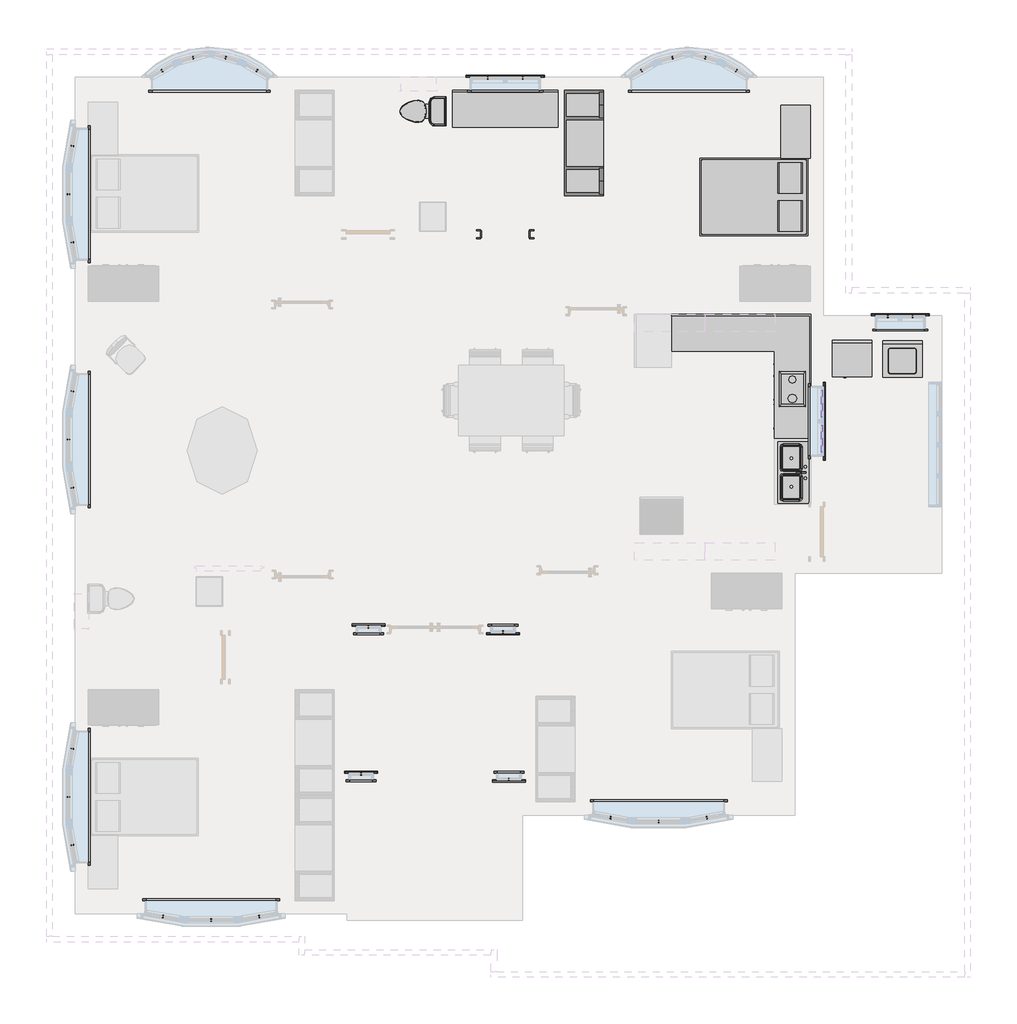
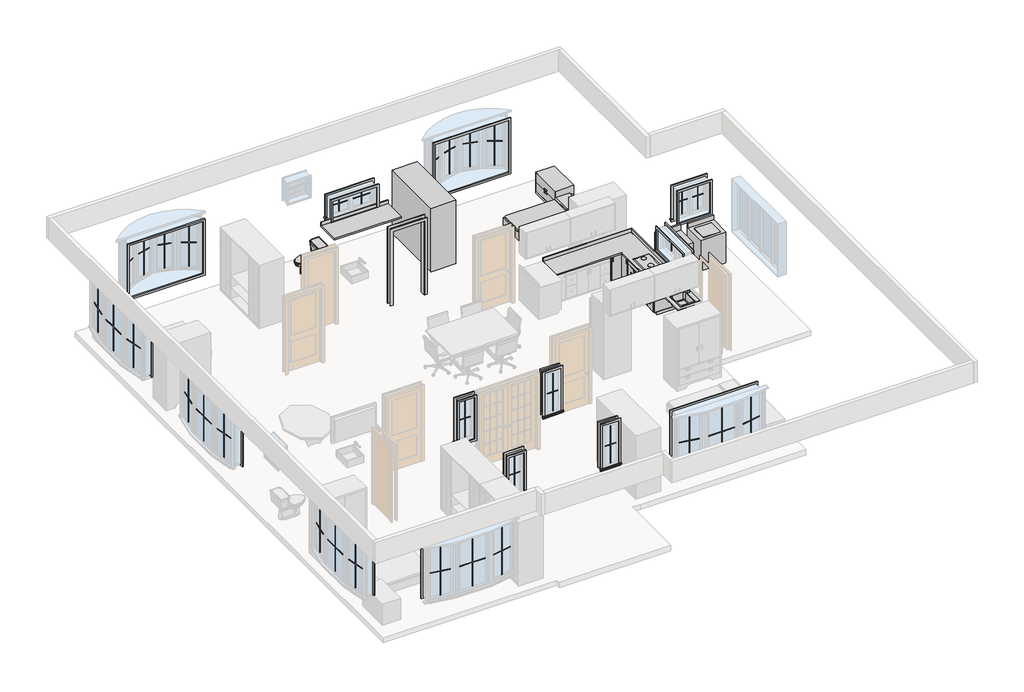
# One storey, part 2 of 2: 58 proxies, 7 furniture elements, 2 flow terminals.
"""IFC4 building model written with IfcOpenShell, lengths in millimetres."""

from ifc_helpers import new_model, si_unit, origin, place, context, project, spatial, transform, mapped, element, save
from components import proxy_3c1fa1d0, proxy_97c73763, muntin_pattern_2x2_muntin_pattern_2x2_d8607f27, muntin_pattern_2x2_muntin_pattern_2x2_395d1e8c, muntin_pattern_2x2_muntin_pattern_2x2_f815d33b, muntin_pattern_2x2_muntin_pattern_2x2_6cb77f41, muntin_pattern_2x2_muntin_pattern_2x2_7d820091, muntin_pattern_2x2_muntin_pattern_2x2_d662aa9d, muntin_pattern_2x2_muntin_pattern_2x2_3e0ecaf2, muntin_pattern_2x2_muntin_pattern_2x2_b3fe6957, muntin_pattern_2x2_muntin_pattern_2x2_0e1f1e2d, proxy_dc468f74, trim_window_exterior_flat_with_sill_a633738d, trim_window_exterior_flat_with_sill_f2223f96, trim_window_exterior_flat_with_sill_499ee38d, trim_window_interior_flat_picture_frame_9ca7b173, trim_window_interior_flat_picture_frame_fb3c0359, trim_window_interior_flat_picture_frame_0870d947, trim_window_interior_flat_picture_frame_1c9020d0, trim_window_interior_flat_picture_frame_a70901f7, proxy_e75280ca, flow_terminal_a53be723, toilet_domestic_3d_toilet_domestic_3d_ba6479b0, toilet_domestic_3d_toilet_domestic_3d_30431060, furniture_b04c6994, furniture_ff3c2f57, furniture_b58f7881, furniture_6b884072, furniture_6990e744, furniture_a71f50c7, furniture_88072bd9

model = new_model("IFC4")

# Units and contexts
model_context = context("Model", 3, world=origin())
ifc_project = project(units=[si_unit("LENGTHUNIT", "METRE", prefix="MILLI")], contexts=[model_context])

# Site, building, storey
site = spatial("IfcSite", under=ifc_project)
building = spatial("IfcBuilding", under=site)
storey = spatial("IfcBuildingStorey", under=building, Elevation=914.4)

# Proxies
placement = place(None, origin())
proxy_shape = proxy_3c1fa1d0(model_context)
element("IfcBuildingElementProxy", 1, Name="Cook Top-2 Unit : 12\" x 18\" 2", ObjectType="Cook Top-2 Unit : 12\" x 18\" 2", at=placement, inside=storey, context=model_context, shape_type="MappedRepresentation", body=[
    mapped(proxy_shape, transform((-7640.9494093, 9917.3485443, 914.4), x_axis=(-1.0, 0.0, 0.0), y_axis=(0.0, -1.0, 0.0), z_axis=(0.0, 0.0, 1.0))),
])
proxy_2_shape = proxy_97c73763(model_context)
element("IfcBuildingElementProxy", 2, Name="Dryer : 27\" x 25\" x 35\"", ObjectType="Dryer : 27\" x 25\" x 35\"", at=placement, inside=storey, context=model_context, shape_type="MappedRepresentation", body=[
    mapped(proxy_2_shape, transform((-7061.0868656, 10105.8627449, 914.4), x_axis=(1.0, 0.0, 0.0), y_axis=(0.0, 1.0, 0.0), z_axis=(0.0, 0.0, 1.0))),
])
muntin_pattern_2x2_muntin_pattern_2x2_shape = muntin_pattern_2x2_muntin_pattern_2x2_d8607f27(model_context)
element("IfcBuildingElementProxy", 3, Name="Muntin Pattern_2x2 : Muntin Pattern_2x2", ObjectType="Muntin Pattern_2x2 : Muntin Pattern_2x2", at=placement, inside=storey, context=model_context, shape_type="MappedRepresentation", body=[
    mapped(muntin_pattern_2x2_muntin_pattern_2x2_shape, transform((-20280.6244093, 13268.4987487, 1644.65), x_axis=(0.0, 1.0, 0.0), y_axis=(-1.0, 0.0, 0.0), z_axis=(0.0, 0.0, 1.0))),
])
element("IfcBuildingElementProxy", 4, Name="Muntin Pattern_2x2 : Muntin Pattern_2x2", ObjectType="Muntin Pattern_2x2 : Muntin Pattern_2x2", at=placement, inside=storey, context=model_context, shape_type="MappedRepresentation", body=[
    mapped(muntin_pattern_2x2_muntin_pattern_2x2_shape, transform((-20280.6244093, 9010.8237487, 1644.65), x_axis=(0.0, 1.0, 0.0), y_axis=(-1.0, 0.0, 0.0), z_axis=(0.0, 0.0, 1.0))),
])
element("IfcBuildingElementProxy", 5, Name="Muntin Pattern_2x2 : Muntin Pattern_2x2", ObjectType="Muntin Pattern_2x2 : Muntin Pattern_2x2", at=placement, inside=storey, context=model_context, shape_type="MappedRepresentation", body=[
    mapped(muntin_pattern_2x2_muntin_pattern_2x2_shape, transform((-20280.6244093, 2810.0487487, 1644.65), x_axis=(0.0, 1.0, 0.0), y_axis=(-1.0, 0.0, 0.0), z_axis=(0.0, 0.0, 1.0))),
])
element("IfcBuildingElementProxy", 6, Name="Muntin Pattern_2x2 : Muntin Pattern_2x2", ObjectType="Muntin Pattern_2x2 : Muntin Pattern_2x2", at=placement, inside=storey, context=model_context, shape_type="MappedRepresentation", body=[
    mapped(muntin_pattern_2x2_muntin_pattern_2x2_shape, transform((-17807.2994093, 670.0987487, 1644.65), x_axis=(-1.0, 0.0, 0.0), y_axis=(0.0, -1.0, 0.0), z_axis=(0.0, 0.0, 1.0))),
])
element("IfcBuildingElementProxy", 7, Name="Muntin Pattern_2x2 : Muntin Pattern_2x2", ObjectType="Muntin Pattern_2x2 : Muntin Pattern_2x2", at=placement, inside=storey, context=model_context, shape_type="MappedRepresentation", body=[
    mapped(muntin_pattern_2x2_muntin_pattern_2x2_shape, transform((-10034.8994093, 2384.5987487, 1644.65), x_axis=(-1.0, 0.0, 0.0), y_axis=(0.0, -1.0, 0.0), z_axis=(0.0, 0.0, 1.0))),
])
muntin_pattern_2x2_muntin_pattern_2x2_2_shape = muntin_pattern_2x2_muntin_pattern_2x2_395d1e8c(model_context)
element("IfcBuildingElementProxy", 8, Name="Muntin Pattern_2x2 : Muntin Pattern_2x2", ObjectType="Muntin Pattern_2x2 : Muntin Pattern_2x2", at=placement, inside=storey, context=model_context, shape_type="MappedRepresentation", body=[
    mapped(muntin_pattern_2x2_muntin_pattern_2x2_2_shape, transform((-20216.0334517, 12432.1293812, 1644.65), x_axis=(-0.1736481776669241, 0.9848077530122091, 0.0), y_axis=(-0.9848077530122091, -0.1736481776669241, 0.0), z_axis=(0.0, 0.0, 1.0))),
])
element("IfcBuildingElementProxy", 9, Name="Muntin Pattern_2x2 : Muntin Pattern_2x2", ObjectType="Muntin Pattern_2x2 : Muntin Pattern_2x2", at=placement, inside=storey, context=model_context, shape_type="MappedRepresentation", body=[
    mapped(muntin_pattern_2x2_muntin_pattern_2x2_2_shape, transform((-20216.0334517, 14104.8681162, 1644.65), x_axis=(0.17364817766693658, 0.984807753012207, 0.0), y_axis=(-0.984807753012207, 0.17364817766693658, 0.0), z_axis=(0.0, 0.0, 1.0))),
])
element("IfcBuildingElementProxy", 10, Name="Muntin Pattern_2x2 : Muntin Pattern_2x2", ObjectType="Muntin Pattern_2x2 : Muntin Pattern_2x2", at=placement, inside=storey, context=model_context, shape_type="MappedRepresentation", body=[
    mapped(muntin_pattern_2x2_muntin_pattern_2x2_2_shape, transform((-20216.0334517, 8174.4543812, 1644.65), x_axis=(-0.1736481776669241, 0.9848077530122091, 0.0), y_axis=(-0.9848077530122091, -0.1736481776669241, 0.0), z_axis=(0.0, 0.0, 1.0))),
])
element("IfcBuildingElementProxy", 11, Name="Muntin Pattern_2x2 : Muntin Pattern_2x2", ObjectType="Muntin Pattern_2x2 : Muntin Pattern_2x2", at=placement, inside=storey, context=model_context, shape_type="MappedRepresentation", body=[
    mapped(muntin_pattern_2x2_muntin_pattern_2x2_2_shape, transform((-20216.0334517, 9847.1931162, 1644.65), x_axis=(0.17364817766693658, 0.984807753012207, 0.0), y_axis=(-0.984807753012207, 0.17364817766693658, 0.0), z_axis=(0.0, 0.0, 1.0))),
])
element("IfcBuildingElementProxy", 12, Name="Muntin Pattern_2x2 : Muntin Pattern_2x2", ObjectType="Muntin Pattern_2x2 : Muntin Pattern_2x2", at=placement, inside=storey, context=model_context, shape_type="MappedRepresentation", body=[
    mapped(muntin_pattern_2x2_muntin_pattern_2x2_2_shape, transform((-20216.0334517, 1973.6793812, 1644.65), x_axis=(-0.1736481776669241, 0.9848077530122091, 0.0), y_axis=(-0.9848077530122091, -0.1736481776669241, 0.0), z_axis=(0.0, 0.0, 1.0))),
])
element("IfcBuildingElementProxy", 13, Name="Muntin Pattern_2x2 : Muntin Pattern_2x2", ObjectType="Muntin Pattern_2x2 : Muntin Pattern_2x2", at=placement, inside=storey, context=model_context, shape_type="MappedRepresentation", body=[
    mapped(muntin_pattern_2x2_muntin_pattern_2x2_2_shape, transform((-20216.0334517, 3646.4181162, 1644.65), x_axis=(0.17364817766693658, 0.984807753012207, 0.0), y_axis=(-0.984807753012207, 0.17364817766693658, 0.0), z_axis=(0.0, 0.0, 1.0))),
])
element("IfcBuildingElementProxy", 14, Name="Muntin Pattern_2x2 : Muntin Pattern_2x2", ObjectType="Muntin Pattern_2x2 : Muntin Pattern_2x2", at=placement, inside=storey, context=model_context, shape_type="MappedRepresentation", body=[
    mapped(muntin_pattern_2x2_muntin_pattern_2x2_2_shape, transform((-16970.9300418, 734.6897062, 1644.65), x_axis=(-0.9848077530122097, -0.1736481776669209, 0.0), y_axis=(0.1736481776669209, -0.9848077530122097, 0.0), z_axis=(0.0, 0.0, 1.0))),
])
element("IfcBuildingElementProxy", 15, Name="Muntin Pattern_2x2 : Muntin Pattern_2x2", ObjectType="Muntin Pattern_2x2 : Muntin Pattern_2x2", at=placement, inside=storey, context=model_context, shape_type="MappedRepresentation", body=[
    mapped(muntin_pattern_2x2_muntin_pattern_2x2_2_shape, transform((-18643.6687768, 734.6897063, 1644.65), x_axis=(-0.9848077530122065, 0.17364817766693977, 0.0), y_axis=(-0.17364817766693977, -0.9848077530122065, 0.0), z_axis=(0.0, 0.0, 1.0))),
])
element("IfcBuildingElementProxy", 16, Name="Muntin Pattern_2x2 : Muntin Pattern_2x2", ObjectType="Muntin Pattern_2x2 : Muntin Pattern_2x2", at=placement, inside=storey, context=model_context, shape_type="MappedRepresentation", body=[
    mapped(muntin_pattern_2x2_muntin_pattern_2x2_2_shape, transform((-9198.5300418, 2449.1897062, 1644.65), x_axis=(-0.9848077530122097, -0.1736481776669209, 0.0), y_axis=(0.1736481776669209, -0.9848077530122097, 0.0), z_axis=(0.0, 0.0, 1.0))),
])
element("IfcBuildingElementProxy", 17, Name="Muntin Pattern_2x2 : Muntin Pattern_2x2", ObjectType="Muntin Pattern_2x2 : Muntin Pattern_2x2", at=placement, inside=storey, context=model_context, shape_type="MappedRepresentation", body=[
    mapped(muntin_pattern_2x2_muntin_pattern_2x2_2_shape, transform((-10871.2687768, 2449.1897063, 1644.65), x_axis=(-0.9848077530122065, 0.17364817766693977, 0.0), y_axis=(-0.17364817766693977, -0.9848077530122065, 0.0), z_axis=(0.0, 0.0, 1.0))),
])
muntin_pattern_2x2_muntin_pattern_2x2_3_shape = muntin_pattern_2x2_muntin_pattern_2x2_f815d33b(model_context)
element("IfcBuildingElementProxy", 18, Name="Muntin Pattern_2x2 : Muntin Pattern_2x2", ObjectType="Muntin Pattern_2x2 : Muntin Pattern_2x2", at=placement, inside=storey, context=model_context, shape_type="MappedRepresentation", body=[
    mapped(muntin_pattern_2x2_muntin_pattern_2x2_3_shape, transform((-18660.5166572, 15411.8794119, 1644.65), x_axis=(0.866025403784444, 0.4999999999999909, 0.0), y_axis=(-0.4999999999999909, 0.866025403784444, 0.0), z_axis=(0.0, 0.0, 1.0))),
])
element("IfcBuildingElementProxy", 19, Name="Muntin Pattern_2x2 : Muntin Pattern_2x2", ObjectType="Muntin Pattern_2x2 : Muntin Pattern_2x2", at=placement, inside=storey, context=model_context, shape_type="MappedRepresentation", body=[
    mapped(muntin_pattern_2x2_muntin_pattern_2x2_3_shape, transform((-18119.7323086, 15635.8687175, 1644.65), x_axis=(0.9659258262890726, 0.2588190451025049, 0.0), y_axis=(-0.2588190451025049, 0.9659258262890726, 0.0), z_axis=(0.0, 0.0, 1.0))),
])
element("IfcBuildingElementProxy", 20, Name="Muntin Pattern_2x2 : Muntin Pattern_2x2", ObjectType="Muntin Pattern_2x2 : Muntin Pattern_2x2", at=placement, inside=storey, context=model_context, shape_type="MappedRepresentation", body=[
    mapped(muntin_pattern_2x2_muntin_pattern_2x2_3_shape, transform((-10335.6666572, 15411.8794119, 1644.65), x_axis=(0.866025403784444, 0.4999999999999909, 0.0), y_axis=(-0.4999999999999909, 0.866025403784444, 0.0), z_axis=(0.0, 0.0, 1.0))),
])
element("IfcBuildingElementProxy", 21, Name="Muntin Pattern_2x2 : Muntin Pattern_2x2", ObjectType="Muntin Pattern_2x2 : Muntin Pattern_2x2", at=placement, inside=storey, context=model_context, shape_type="MappedRepresentation", body=[
    mapped(muntin_pattern_2x2_muntin_pattern_2x2_3_shape, transform((-9794.8823086, 15635.8687175, 1644.65), x_axis=(0.9659258262890726, 0.2588190451025049, 0.0), y_axis=(-0.2588190451025049, 0.9659258262890726, 0.0), z_axis=(0.0, 0.0, 1.0))),
])
muntin_pattern_2x2_muntin_pattern_2x2_4_shape = muntin_pattern_2x2_muntin_pattern_2x2_6cb77f41(model_context)
element("IfcBuildingElementProxy", 22, Name="Muntin Pattern_2x2 : Muntin Pattern_2x2", ObjectType="Muntin Pattern_2x2 : Muntin Pattern_2x2", at=placement, inside=storey, context=model_context, shape_type="MappedRepresentation", body=[
    mapped(muntin_pattern_2x2_muntin_pattern_2x2_4_shape, transform((-17011.2321614, 15411.8794119, 1644.65), x_axis=(-0.8660254037844407, 0.49999999999999656, 0.0), y_axis=(-0.49999999999999656, -0.8660254037844407, 0.0), z_axis=(0.0, 0.0, 1.0))),
])
element("IfcBuildingElementProxy", 23, Name="Muntin Pattern_2x2 : Muntin Pattern_2x2", ObjectType="Muntin Pattern_2x2 : Muntin Pattern_2x2", at=placement, inside=storey, context=model_context, shape_type="MappedRepresentation", body=[
    mapped(muntin_pattern_2x2_muntin_pattern_2x2_4_shape, transform((-17552.01651, 15635.8687176, 1644.65), x_axis=(-0.9659258262890709, 0.25881904510251125, 0.0), y_axis=(-0.25881904510251125, -0.9659258262890709, 0.0), z_axis=(0.0, 0.0, 1.0))),
])
element("IfcBuildingElementProxy", 24, Name="Muntin Pattern_2x2 : Muntin Pattern_2x2", ObjectType="Muntin Pattern_2x2 : Muntin Pattern_2x2", at=placement, inside=storey, context=model_context, shape_type="MappedRepresentation", body=[
    mapped(muntin_pattern_2x2_muntin_pattern_2x2_4_shape, transform((-8686.3821614, 15411.8794119, 1644.65), x_axis=(-0.8660254037844407, 0.49999999999999656, 0.0), y_axis=(-0.49999999999999656, -0.8660254037844407, 0.0), z_axis=(0.0, 0.0, 1.0))),
])
element("IfcBuildingElementProxy", 25, Name="Muntin Pattern_2x2 : Muntin Pattern_2x2", ObjectType="Muntin Pattern_2x2 : Muntin Pattern_2x2", at=placement, inside=storey, context=model_context, shape_type="MappedRepresentation", body=[
    mapped(muntin_pattern_2x2_muntin_pattern_2x2_4_shape, transform((-9227.16651, 15635.8687176, 1644.65), x_axis=(-0.9659258262890709, 0.25881904510251125, 0.0), y_axis=(-0.25881904510251125, -0.9659258262890709, 0.0), z_axis=(0.0, 0.0, 1.0))),
])
muntin_pattern_2x2_muntin_pattern_2x2_5_shape = muntin_pattern_2x2_muntin_pattern_2x2_7d820091(model_context)
element("IfcBuildingElementProxy", 26, Name="Muntin Pattern_2x2 : Muntin Pattern_2x2", ObjectType="Muntin Pattern_2x2 : Muntin Pattern_2x2", at=placement, inside=storey, context=model_context, shape_type="MappedRepresentation", body=[
    mapped(muntin_pattern_2x2_muntin_pattern_2x2_5_shape, transform((-13005.1119093, 15287.7987487, 1898.65), x_axis=(1.0, 0.0, 0.0), y_axis=(0.0, 1.0, 0.0), z_axis=(0.0, 0.0, 1.0))),
])
element("IfcBuildingElementProxy", 27, Name="Muntin Pattern_2x2 : Muntin Pattern_2x2", ObjectType="Muntin Pattern_2x2 : Muntin Pattern_2x2", at=placement, inside=storey, context=model_context, shape_type="MappedRepresentation", body=[
    mapped(muntin_pattern_2x2_muntin_pattern_2x2_5_shape, transform((-7186.9244093, 9631.5362487, 2139.95), x_axis=(0.0, -1.0, 0.0), y_axis=(1.0, 0.0, 0.0), z_axis=(0.0, 0.0, 1.0))),
])
muntin_pattern_2x2_muntin_pattern_2x2_6_shape = muntin_pattern_2x2_muntin_pattern_2x2_d662aa9d(model_context)
element("IfcBuildingElementProxy", 28, Name="Muntin Pattern_2x2 : Muntin Pattern_2x2", ObjectType="Muntin Pattern_2x2 : Muntin Pattern_2x2", at=placement, inside=storey, context=model_context, shape_type="MappedRepresentation", body=[
    mapped(muntin_pattern_2x2_muntin_pattern_2x2_6_shape, transform((-12398.6869093, 15287.7987487, 1898.65), x_axis=(-1.0, 0.0, 0.0), y_axis=(0.0, -1.0, 0.0), z_axis=(0.0, 0.0, 1.0))),
])
element("IfcBuildingElementProxy", 29, Name="Muntin Pattern_2x2 : Muntin Pattern_2x2", ObjectType="Muntin Pattern_2x2 : Muntin Pattern_2x2", at=placement, inside=storey, context=model_context, shape_type="MappedRepresentation", body=[
    mapped(muntin_pattern_2x2_muntin_pattern_2x2_6_shape, transform((-7186.9244093, 9025.1112487, 2139.95), x_axis=(0.0, 1.0, 0.0), y_axis=(-1.0, 0.0, 0.0), z_axis=(0.0, 0.0, 1.0))),
])
muntin_pattern_2x2_muntin_pattern_2x2_7_shape = muntin_pattern_2x2_muntin_pattern_2x2_3e0ecaf2(model_context)
element("IfcBuildingElementProxy", 30, Name="Muntin Pattern_2x2 : Muntin Pattern_2x2", ObjectType="Muntin Pattern_2x2 : Muntin Pattern_2x2", at=placement, inside=storey, context=model_context, shape_type="MappedRepresentation", body=[
    mapped(muntin_pattern_2x2_muntin_pattern_2x2_7_shape, transform((-5629.5869093, 11147.5987487, 1898.65), x_axis=(-1.0, 0.0, 0.0), y_axis=(0.0, -1.0, 0.0), z_axis=(0.0, 0.0, 1.0))),
])
muntin_pattern_2x2_muntin_pattern_2x2_8_shape = muntin_pattern_2x2_muntin_pattern_2x2_b3fe6957(model_context)
element("IfcBuildingElementProxy", 31, Name="Muntin Pattern_2x2 : Muntin Pattern_2x2", ObjectType="Muntin Pattern_2x2 : Muntin Pattern_2x2", at=placement, inside=storey, context=model_context, shape_type="MappedRepresentation", body=[
    mapped(muntin_pattern_2x2_muntin_pattern_2x2_8_shape, transform((-6058.2119093, 11147.5987487, 1898.65), x_axis=(1.0, 0.0, 0.0), y_axis=(0.0, 1.0, 0.0), z_axis=(0.0, 0.0, 1.0))),
])
muntin_pattern_2x2_muntin_pattern_2x2_9_shape = muntin_pattern_2x2_muntin_pattern_2x2_0e1f1e2d(model_context)
element("IfcBuildingElementProxy", 32, Name="Muntin Pattern_2x2 : Muntin Pattern_2x2", ObjectType="Muntin Pattern_2x2 : Muntin Pattern_2x2", at=placement, inside=storey, context=model_context, shape_type="MappedRepresentation", body=[
    mapped(muntin_pattern_2x2_muntin_pattern_2x2_9_shape, transform((-12638.3994093, 3114.8487487, 1898.65), x_axis=(-1.0, 0.0, 0.0), y_axis=(0.0, -1.0, 0.0), z_axis=(0.0, 0.0, 1.0))),
])
element("IfcBuildingElementProxy", 33, Name="Muntin Pattern_2x2 : Muntin Pattern_2x2", ObjectType="Muntin Pattern_2x2 : Muntin Pattern_2x2", at=placement, inside=storey, context=model_context, shape_type="MappedRepresentation", body=[
    mapped(muntin_pattern_2x2_muntin_pattern_2x2_9_shape, transform((-15203.7994093, 3210.0987487, 1898.65), x_axis=(1.0, 0.0, 0.0), y_axis=(0.0, 1.0, 0.0), z_axis=(0.0, 0.0, 1.0))),
])
element("IfcBuildingElementProxy", 34, Name="Muntin Pattern_2x2 : Muntin Pattern_2x2", ObjectType="Muntin Pattern_2x2 : Muntin Pattern_2x2", at=placement, inside=storey, context=model_context, shape_type="MappedRepresentation", body=[
    mapped(muntin_pattern_2x2_muntin_pattern_2x2_9_shape, transform((-15076.7994093, 5762.7987487, 1898.65), x_axis=(1.0, 0.0, 0.0), y_axis=(0.0, 1.0, 0.0), z_axis=(0.0, 0.0, 1.0))),
])
element("IfcBuildingElementProxy", 35, Name="Muntin Pattern_2x2 : Muntin Pattern_2x2", ObjectType="Muntin Pattern_2x2 : Muntin Pattern_2x2", at=placement, inside=storey, context=model_context, shape_type="MappedRepresentation", body=[
    mapped(muntin_pattern_2x2_muntin_pattern_2x2_9_shape, transform((-12739.9994093, 5667.5487487, 1898.65), x_axis=(-1.0, 0.0, 0.0), y_axis=(0.0, -1.0, 0.0), z_axis=(0.0, 0.0, 1.0))),
])
proxy_3_shape = proxy_dc468f74(model_context)
element("IfcBuildingElementProxy", 36, Name="Passage Opening-Cased : 34\" x 84\"", ObjectType="Passage Opening-Cased : 34\" x 84\"", at=placement, inside=storey, context=model_context, shape_type="MappedRepresentation", body=[
    mapped(proxy_3_shape, transform((-12693.7107526, 12573.1737487, 914.4), x_axis=(1.0, 0.0, 0.0), y_axis=(0.0, 1.0, 0.0), z_axis=(0.0, 0.0, 1.0))),
])
trim_window_exterior_flat_with_sill_shape = trim_window_exterior_flat_with_sill_a633738d(model_context)
element("IfcBuildingElementProxy", 37, Name="Trim-Window-Exterior-Flat : with Sill", ObjectType="Trim-Window-Exterior-Flat : with Sill", at=placement, inside=storey, context=model_context, shape_type="MappedRepresentation", body=[
    mapped(trim_window_exterior_flat_with_sill_shape, transform((-12701.8994093, 15297.3237487, 2438.4), x_axis=(-1.0, 0.0, 0.0), y_axis=(0.0, 0.0, 1.0), z_axis=(0.0, 1.0, 0.0))),
])
element("IfcBuildingElementProxy", 38, Name="Trim-Window-Exterior-Flat : with Sill", ObjectType="Trim-Window-Exterior-Flat : with Sill", at=placement, inside=storey, context=model_context, shape_type="MappedRepresentation", body=[
    mapped(trim_window_exterior_flat_with_sill_shape, transform((-7177.3994093, 9328.3237487, 2679.7), x_axis=(0.0, 1.0, 0.0), y_axis=(0.0, 0.0, 1.0), z_axis=(1.0, 0.0, 0.0))),
])
trim_window_exterior_flat_with_sill_2_shape = trim_window_exterior_flat_with_sill_f2223f96(model_context)
element("IfcBuildingElementProxy", 39, Name="Trim-Window-Exterior-Flat : with Sill", ObjectType="Trim-Window-Exterior-Flat : with Sill", at=placement, inside=storey, context=model_context, shape_type="MappedRepresentation", body=[
    mapped(trim_window_exterior_flat_with_sill_2_shape, transform((-5843.8994093, 11157.1237487, 2743.2), x_axis=(1.0, 0.0, 0.0), y_axis=(0.0, 0.0, -1.0), z_axis=(0.0, 1.0, 0.0))),
])
trim_window_exterior_flat_with_sill_3_shape = trim_window_exterior_flat_with_sill_499ee38d(model_context)
element("IfcBuildingElementProxy", 40, Name="Trim-Window-Exterior-Flat : with Sill", ObjectType="Trim-Window-Exterior-Flat : with Sill", at=placement, inside=storey, context=model_context, shape_type="MappedRepresentation", body=[
    mapped(trim_window_exterior_flat_with_sill_3_shape, transform((-12638.3994093, 3105.3237487, 3048.0), x_axis=(1.0, 0.0, 0.0), y_axis=(0.0, 0.0, 1.0), z_axis=(0.0, -1.0, 0.0))),
])
element("IfcBuildingElementProxy", 41, Name="Trim-Window-Exterior-Flat : with Sill", ObjectType="Trim-Window-Exterior-Flat : with Sill", at=placement, inside=storey, context=model_context, shape_type="MappedRepresentation", body=[
    mapped(trim_window_exterior_flat_with_sill_3_shape, transform((-15203.7994093, 3219.6237487, 3048.0), x_axis=(-1.0, 0.0, 0.0), y_axis=(0.0, 0.0, 1.0), z_axis=(0.0, 1.0, 0.0))),
])
element("IfcBuildingElementProxy", 42, Name="Trim-Window-Exterior-Flat : with Sill", ObjectType="Trim-Window-Exterior-Flat : with Sill", at=placement, inside=storey, context=model_context, shape_type="MappedRepresentation", body=[
    mapped(trim_window_exterior_flat_with_sill_3_shape, transform((-15076.7994093, 5772.3237487, 3048.0), x_axis=(-1.0, 0.0, 0.0), y_axis=(0.0, 0.0, 1.0), z_axis=(0.0, 1.0, 0.0))),
])
element("IfcBuildingElementProxy", 43, Name="Trim-Window-Exterior-Flat : with Sill", ObjectType="Trim-Window-Exterior-Flat : with Sill", at=placement, inside=storey, context=model_context, shape_type="MappedRepresentation", body=[
    mapped(trim_window_exterior_flat_with_sill_3_shape, transform((-12739.9994093, 5658.0237487, 3048.0), x_axis=(1.0, 0.0, 0.0), y_axis=(0.0, 0.0, 1.0), z_axis=(0.0, -1.0, 0.0))),
])
trim_window_interior_flat_picture_frame_shape = trim_window_interior_flat_picture_frame_9ca7b173(model_context)
element("IfcBuildingElementProxy", 44, Name="Trim-Window-Interior-Flat : Picture Frame", ObjectType="Trim-Window-Interior-Flat : Picture Frame", at=placement, inside=storey, context=model_context, shape_type="MappedRepresentation", body=[
    mapped(trim_window_interior_flat_picture_frame_shape, transform((-19940.8994093, 13268.4987487, 3098.8), x_axis=(0.0, 1.0, 0.0), y_axis=(0.0, 0.0, 1.0), z_axis=(1.0, 0.0, 0.0))),
])
element("IfcBuildingElementProxy", 45, Name="Trim-Window-Interior-Flat : Picture Frame", ObjectType="Trim-Window-Interior-Flat : Picture Frame", at=placement, inside=storey, context=model_context, shape_type="MappedRepresentation", body=[
    mapped(trim_window_interior_flat_picture_frame_shape, transform((-19940.8994093, 9010.8237487, 3098.8), x_axis=(0.0, 1.0, 0.0), y_axis=(0.0, 0.0, 1.0), z_axis=(1.0, 0.0, 0.0))),
])
element("IfcBuildingElementProxy", 46, Name="Trim-Window-Interior-Flat : Picture Frame", ObjectType="Trim-Window-Interior-Flat : Picture Frame", at=placement, inside=storey, context=model_context, shape_type="MappedRepresentation", body=[
    mapped(trim_window_interior_flat_picture_frame_shape, transform((-19940.8994093, 2810.0487487, 3098.8), x_axis=(0.0, 1.0, 0.0), y_axis=(0.0, 0.0, 1.0), z_axis=(1.0, 0.0, 0.0))),
])
element("IfcBuildingElementProxy", 47, Name="Trim-Window-Interior-Flat : Picture Frame", ObjectType="Trim-Window-Interior-Flat : Picture Frame", at=placement, inside=storey, context=model_context, shape_type="MappedRepresentation", body=[
    mapped(trim_window_interior_flat_picture_frame_shape, transform((-17807.2994093, 1009.8237487, 3098.8), x_axis=(-1.0, 0.0, 0.0), y_axis=(0.0, 0.0, 1.0), z_axis=(0.0, 1.0, 0.0))),
])
element("IfcBuildingElementProxy", 48, Name="Trim-Window-Interior-Flat : Picture Frame", ObjectType="Trim-Window-Interior-Flat : Picture Frame", at=placement, inside=storey, context=model_context, shape_type="MappedRepresentation", body=[
    mapped(trim_window_interior_flat_picture_frame_shape, transform((-10034.8994093, 2724.3237487, 3098.8), x_axis=(-1.0, 0.0, 0.0), y_axis=(0.0, 0.0, 1.0), z_axis=(0.0, 1.0, 0.0))),
])
trim_window_interior_flat_picture_frame_2_shape = trim_window_interior_flat_picture_frame_fb3c0359(model_context)
element("IfcBuildingElementProxy", 49, Name="Trim-Window-Interior-Flat : Picture Frame", ObjectType="Trim-Window-Interior-Flat : Picture Frame", at=placement, inside=storey, context=model_context, shape_type="MappedRepresentation", body=[
    mapped(trim_window_interior_flat_picture_frame_2_shape, transform((-17835.8744093, 15068.7237487, 3098.8), x_axis=(1.0, 0.0, 0.0), y_axis=(0.0, 0.0, 1.0), z_axis=(0.0, -1.0, 0.0))),
])
element("IfcBuildingElementProxy", 50, Name="Trim-Window-Interior-Flat : Picture Frame", ObjectType="Trim-Window-Interior-Flat : Picture Frame", at=placement, inside=storey, context=model_context, shape_type="MappedRepresentation", body=[
    mapped(trim_window_interior_flat_picture_frame_2_shape, transform((-9511.0244093, 15068.7237487, 3098.8), x_axis=(1.0, 0.0, 0.0), y_axis=(0.0, 0.0, 1.0), z_axis=(0.0, -1.0, 0.0))),
])
trim_window_interior_flat_picture_frame_3_shape = trim_window_interior_flat_picture_frame_0870d947(model_context)
element("IfcBuildingElementProxy", 51, Name="Trim-Window-Interior-Flat : Picture Frame", ObjectType="Trim-Window-Interior-Flat : Picture Frame", at=placement, inside=storey, context=model_context, shape_type="MappedRepresentation", body=[
    mapped(trim_window_interior_flat_picture_frame_3_shape, transform((-12701.8994093, 15068.7237487, 2438.4), x_axis=(1.0, 0.0, 0.0), y_axis=(0.0, 0.0, 1.0), z_axis=(0.0, -1.0, 0.0))),
])
element("IfcBuildingElementProxy", 52, Name="Trim-Window-Interior-Flat : Picture Frame", ObjectType="Trim-Window-Interior-Flat : Picture Frame", at=placement, inside=storey, context=model_context, shape_type="MappedRepresentation", body=[
    mapped(trim_window_interior_flat_picture_frame_3_shape, transform((-7405.9994093, 9328.3237487, 2679.7), x_axis=(0.0, -1.0, 0.0), y_axis=(0.0, 0.0, 1.0), z_axis=(-1.0, 0.0, 0.0))),
])
trim_window_interior_flat_picture_frame_4_shape = trim_window_interior_flat_picture_frame_1c9020d0(model_context)
element("IfcBuildingElementProxy", 53, Name="Trim-Window-Interior-Flat : Picture Frame", ObjectType="Trim-Window-Interior-Flat : Picture Frame", at=placement, inside=storey, context=model_context, shape_type="MappedRepresentation", body=[
    mapped(trim_window_interior_flat_picture_frame_4_shape, transform((-5843.8994093, 10928.5237487, 2743.2), x_axis=(-1.0, 0.0, 0.0), y_axis=(0.0, 0.0, -1.0), z_axis=(0.0, -1.0, 0.0))),
])
trim_window_interior_flat_picture_frame_5_shape = trim_window_interior_flat_picture_frame_a70901f7(model_context)
element("IfcBuildingElementProxy", 54, Name="Trim-Window-Interior-Flat : Picture Frame", ObjectType="Trim-Window-Interior-Flat : Picture Frame", at=placement, inside=storey, context=model_context, shape_type="MappedRepresentation", body=[
    mapped(trim_window_interior_flat_picture_frame_5_shape, transform((-12638.3994093, 3219.6237487, 3048.0), x_axis=(-1.0, 0.0, 0.0), y_axis=(0.0, 0.0, 1.0), z_axis=(0.0, 1.0, 0.0))),
])
element("IfcBuildingElementProxy", 55, Name="Trim-Window-Interior-Flat : Picture Frame", ObjectType="Trim-Window-Interior-Flat : Picture Frame", at=placement, inside=storey, context=model_context, shape_type="MappedRepresentation", body=[
    mapped(trim_window_interior_flat_picture_frame_5_shape, transform((-15203.7994093, 3105.3237487, 3048.0), x_axis=(1.0, 0.0, 0.0), y_axis=(0.0, 0.0, 1.0), z_axis=(0.0, -1.0, 0.0))),
])
element("IfcBuildingElementProxy", 56, Name="Trim-Window-Interior-Flat : Picture Frame", ObjectType="Trim-Window-Interior-Flat : Picture Frame", at=placement, inside=storey, context=model_context, shape_type="MappedRepresentation", body=[
    mapped(trim_window_interior_flat_picture_frame_5_shape, transform((-15076.7994093, 5658.0237487, 3048.0), x_axis=(1.0, 0.0, 0.0), y_axis=(0.0, 0.0, 1.0), z_axis=(0.0, -1.0, 0.0))),
])
element("IfcBuildingElementProxy", 57, Name="Trim-Window-Interior-Flat : Picture Frame", ObjectType="Trim-Window-Interior-Flat : Picture Frame", at=placement, inside=storey, context=model_context, shape_type="MappedRepresentation", body=[
    mapped(trim_window_interior_flat_picture_frame_5_shape, transform((-12739.9994093, 5772.3237487, 3048.0), x_axis=(-1.0, 0.0, 0.0), y_axis=(0.0, 0.0, 1.0), z_axis=(0.0, 1.0, 0.0))),
])
proxy_4_shape = proxy_e75280ca(model_context)
element("IfcBuildingElementProxy", 58, Name="Washer : 27\" x 25\" x 35\"", ObjectType="Washer : 27\" x 25\" x 35\"", at=placement, inside=storey, context=model_context, shape_type="MappedRepresentation", body=[
    mapped(proxy_4_shape, transform((-6225.1498445, 10127.1062802, 914.4), x_axis=(1.0, 0.0, 0.0), y_axis=(0.0, 1.0, 0.0), z_axis=(0.0, 0.0, 1.0))),
])

# Flow terminals
flow_terminal_shape = flow_terminal_a53be723(model_context)
element("IfcFlowTerminal", 59, ObjectType="Sink Kitchen-Double : 42\" x 21\"", at=placement, inside=storey, context=model_context, shape_type="MappedRepresentation", body=[
    mapped(flow_terminal_shape, transform((-7700.4448104, 8455.0129893, 914.4), x_axis=(0.0, -1.0, 0.0), y_axis=(1.0, 0.0, 0.0), z_axis=(0.0, 0.0, 1.0))),
])
toilet_domestic_3d_toilet_domestic_3d_shape = toilet_domestic_3d_toilet_domestic_3d_ba6479b0(model_context)
toilet_domestic_3d_toilet_domestic_3d_2_shape = toilet_domestic_3d_toilet_domestic_3d_30431060(model_context)
element("IfcFlowTerminal", 60, ObjectType="Toilet-Domestic-3D : Toilet-Domestic-3D", at=placement, inside=storey, context=model_context, shape_type="MappedRepresentation", body=[
    mapped(toilet_domestic_3d_toilet_domestic_3d_shape, transform((-14225.2954366, 14706.7737487, 914.4), x_axis=(0.0, -1.0, 0.0), y_axis=(1.0, 0.0, 0.0), z_axis=(0.0, 0.0, 1.0))),
    mapped(toilet_domestic_3d_toilet_domestic_3d_2_shape, transform((-14225.2954366, 14706.7737487, 914.4), x_axis=(0.0, -1.0, 0.0), y_axis=(1.0, 0.0, 0.0), z_axis=(0.0, 0.0, 1.0))),
])

# Furniture
furniture_shape = furniture_b04c6994(model_context)
element("IfcFurniture", 61, ObjectType="48\" 2", at=placement, inside=storey, context=model_context, shape_type="MappedRepresentation", body=[
    mapped(furniture_shape, transform((-7405.9994093, 9749.3687087, 914.4), x_axis=(0.0, -1.0, 0.0), y_axis=(1.0, 0.0, 0.0), z_axis=(0.0, 0.0, 1.0))),
])
furniture_2_shape = furniture_ff3c2f57(model_context)
element("IfcFurniture", 62, ObjectType="Base Cabinet-Corner Unit-Square : 36\" 2", at=placement, inside=storey, context=model_context, shape_type="MappedRepresentation", body=[
    mapped(furniture_2_shape, transform((-7932.7371142, 11182.5237487, 914.4), x_axis=(1.0, 0.0, 0.0), y_axis=(0.0, 1.0, 0.0), z_axis=(0.0, 0.0, 1.0))),
])
furniture_3_shape = furniture_b58f7881(model_context)
element("IfcFurniture", 63, ObjectType="Bed-Box : Double 53\" x 74\"", at=placement, inside=storey, context=model_context, shape_type="MappedRepresentation", body=[
    mapped(furniture_3_shape, transform((-8149.4699011, 13560.0262077, 914.4), x_axis=(0.0, -1.0, 0.0), y_axis=(1.0, 0.0, 0.0), z_axis=(0.0, 0.0, 1.0))),
])
furniture_4_shape = furniture_6b884072(model_context)
element("IfcFurniture", 64, ObjectType="Cabinet File-Lateral 2 Drawer : 36\" x 20\" x 24\"", at=placement, inside=storey, context=model_context, shape_type="MappedRepresentation", body=[
    mapped(furniture_4_shape, transform((-6725.6810332, 14171.1512348, 914.4), x_axis=(0.0, -1.0, 0.0), y_axis=(1.0, 0.0, 0.0), z_axis=(0.0, 0.0, 1.0))),
])
furniture_5_shape = furniture_6990e744(model_context)
element("IfcFurniture", 65, ObjectType="Counter Top : 24\" Depth", at=placement, inside=storey, context=model_context, shape_type="MappedRepresentation", body=[
    mapped(furniture_5_shape, transform((-12415.8371142, 15068.7237487, 914.4), x_axis=(1.0, 0.0, 0.0), y_axis=(0.0, 1.0, 0.0), z_axis=(0.0, 0.0, 1.0))),
])
furniture_6_shape = furniture_a71f50c7(model_context)
element("IfcFurniture", 66, ObjectType="Counter Top-L Shaped : 24\" Depth", at=placement, inside=storey, context=model_context, shape_type="MappedRepresentation", body=[
    mapped(furniture_6_shape, transform((-7393.2994093, 9982.0614536, 914.4), x_axis=(0.0, -1.0, 0.0), y_axis=(1.0, 0.0, 0.0), z_axis=(0.0, 0.0, 1.0))),
])
furniture_7_shape = furniture_88072bd9(model_context)
element("IfcFurniture", 67, ObjectType="Entertainment Center.0001 : 72\" x 72\" x 24\"", at=placement, inside=storey, context=model_context, shape_type="MappedRepresentation", body=[
    mapped(furniture_7_shape, transform((-11774.7994093, 14154.3237487, 914.4), x_axis=(0.0, 1.0, 0.0), y_axis=(-1.0, 0.0, 0.0), z_axis=(0.0, 0.0, 1.0))),
])

save(model, "model.ifc")

# Revit data of these elements
# Type "Cook Top-2 Unit : 12\" x 18\" 2"
#   Assembly Code = "E1090400"
#   Counter Height = 3' - 0"
#   Depth = 2' - 0"
#   Width = 1' - 6"
#   Burner Material = Metal - Chrome
#   Cooktop Material = Metal - Steel, Polished
#   Default Elevation = 0
# Type "Dryer : 27\" x 25\" x 35\""
#   Label = "D"
#   Assembly Code = "E1090400"
#   Depth = 2' - 1"
#   Height = 2' - 11"
#   Width = 2' - 3"
#   Dryer Material = Metal - Paint Finish - Ivory,Glossy
#   Default Elevation = 0
# Type "Muntin Pattern_2x2 : Muntin Pattern_2x2"
#   Width [instance default] = 4' - 0"
#   Thickness = 0' - 0 1/2"
#   Height [instance default] = 4' - 0"
#   Distance = 0' - 0 3/4"
#   Interior Material [instance default] = none
#   Exterior Material [instance default] = none
#   Default Elevation = 0
# Type "Passage Opening-Cased : 34\" x 84\""
#   Height = 7' - 0"
#   Trim Thickness = 0' - 0 3/4"
#   Trim Width = 0' - 3"
#   Width = 2' - 10"
#   Frame Material = Door - Frame
#   Default Elevation = 0
# Type "Trim-Window-Exterior-Flat : with Sill"
#   Trim Width = 0' - 2 1/4"
#   Trim Thickness_Picture Frame = 0' - 1 1/4"
#   Trim Thickness_with Sill = 0' - 0 3/4"
#   Sill Thickness = 0' - 1 1/4"
#   Opening Width [instance default] = 2' - 0"
#   Opening Height [instance default] = 3' - 0"
#   Default Elevation = 4' - 0"
#   Sill = yes
#   Picture Frame = no
#   Trim Material [instance default] = none
# Type "Trim-Window-Interior-Flat : Picture Frame"
#   Trim Thickness_Picture Frame = 0' - 1 1/4"
#   Trim Width = 0' - 2 1/4"
#   Trim Thickness_with Sill = 0' - 0 3/4"
#   Sill Thickness = 0' - 1 1/4"
#   Opening Width [instance default] = 2' - 0"
#   Opening Height [instance default] = 3' - 0"
#   Default Elevation = 4' - 0"
#   Sill = no
#   Picture Frame = yes
#   Trim Material [instance default] = none
# Type "Washer : 27\" x 25\" x 35\""
#   Label = "W"
#   Assembly Code = "E1090400"
#   Depth = 2' - 1"
#   Height = 2' - 11"
#   Width = 2' - 3"
#   Washer Material = Metal - Paint Finish - Ivory,Matte
#   Default Elevation = 0
# Type "Sink Kitchen-Double : 42\" x 21\""
#   Assembly Code = "D2010410"
#   Counter Height = 3' - 0"
#   Depth = 1' - 9"
#   Width = 3' - 6"
#   Faucet Material = Steel, Polished
#   Sink Material = Steel, Polished
#   Default Elevation = 0
# Type "Toilet-Domestic-3D : Toilet-Domestic-3D"
#   Assembly Code = "D2010110"
#   Toilet - Bowl/Basin Material = Porcelain, Linen
#   Toilet - Seat Material = Laminate, Linen, Matte
#   Default Elevation = 0
# Type "48\" 2"
#   Assembly Code = "C1030410"
#   Depth = 2' - 0"
#   Height = 2' - 11 1/2"
#   Toe Depth = 0' - 3"
#   Toe Height = 0' - 3 1/2"
#   Width = 4' - 0"
#   Cabinet Material = none
#   Door/Drawer Material = none
#   Handle Material = Cabinets - Handles
#   Default Elevation = 0
# Type "Base Cabinet-Corner Unit-Square : 36\" 2"
#   Assembly Code = "C1030410"
#   Depth = 2' - 0"
#   Height = 2' - 11 1/2"
#   Toe Depth = 0' - 3"
#   Toe Height = 0' - 3 1/2"
#   Width = 3' - 0"
#   Cabinet Material = Cabinets
#   Door/Drawer Material = Cabinets
#   Handle Material = Cabinets - Handles
#   Default Elevation = 0
# Type "Bed-Box : Double 53\" x 74\""
#   Assembly Code = "E2020200"
#   Length = 6' - 2"
#   Width = 4' - 5"
#   Frame Material = Birch
#   Mattress Material = Linen, White
#   Default Elevation = 0
# Type "Cabinet File-Lateral 2 Drawer : 36\" x 20\" x 24\""
#   Assembly Code = "E2020200"
#   Depth = 1' - 8"
#   Height = 2' - 0"
#   Width = 3' - 0"
#   Material = Metal - Steel
#   Default Elevation = 0
# Type "Counter Top : 24\" Depth"
#   Assembly Code = "C1030400"
#   Counter Thickness = 0' - 1 1/2"
#   Depth = 2' - 1"
#   Height = 3' - 0"
#   Length [instance default] = 8' - 0"
#   Counter Top Material = none
#   Default Elevation = 0
# Type "Counter Top-L Shaped : 24\" Depth"
#   Assembly Code = "C1030400"
#   Counter Thickness = 0' - 1 1/2"
#   Depth = 2' - 1"
#   Height = 3' - 0"
#   Length - Leg 1 [instance default] = 8' - 0"
#   Length - Leg 2 [instance default] = 6' - 0"
#   Counter Top Material = none
#   Default Elevation = 0
# Type "Entertainment Center.0001 : 72\" x 72\" x 24\""
#   Assembly Code = "E2020200"
#   Center Width = 2' - 8"
#   Depth = 2' - 0"
#   Height = 6' - 0"
#   Width = 6' - 0"
#   Material = none
#   Default Elevation = 0
# Element 1 (IfcBuildingElementProxy, "Cook Top-2 Unit : 12\" x 18\" 2")
#   Phase Created = New Construction
#   Materials on its faces: "Metal - Steel, Polished", "Metal - Chrome"
# Element 2 (IfcBuildingElementProxy, "Dryer : 27\" x 25\" x 35\"")
#   Phase Created = New Construction
#   Materials on its faces: "Metal - Paint Finish - Ivory,Glossy"
# Elements 3, 4, 5, 6, 7 (IfcBuildingElementProxy, "Muntin Pattern_2x2 : Muntin Pattern_2x2")
#   Width = 2' - 3.57789"
#   Height = 4' - 6 1/2"
#   Interior Material = Wood - Stained
#   Exterior Material = Clad - White
#   Phase Created = New Construction
#   Materials on its faces: "Clad - White", "Wood - Stained"
# Elements 8, 9, 10, 11, 12, 13, 14, 15, 16, 17 (IfcBuildingElementProxy, "Muntin Pattern_2x2 : Muntin Pattern_2x2")
#   Width = 1' - 7.85416"
#   Height = 4' - 6 1/2"
#   Interior Material = Wood - Stained
#   Exterior Material = Clad - White
#   Phase Created = New Construction
#   Materials on its faces: "Clad - White", "Wood - Stained"
# Elements 18, 19, 20, 21, 22, 23, 24, 25 (IfcBuildingElementProxy, "Muntin Pattern_2x2 : Muntin Pattern_2x2")
#   Width = 1' - 1.8393"
#   Height = 4' - 6 1/2"
#   Interior Material = Wood - Stained
#   Exterior Material = Clad - White
#   Phase Created = New Construction
#   Materials on its faces: "Clad - White", "Wood - Stained"
# Elements 26, 27, 28, 29 (IfcBuildingElementProxy, "Muntin Pattern_2x2 : Muntin Pattern_2x2")
#   Width = 1' - 6 5/8"
#   Height = 1' - 6 1/2"
#   Interior Material = Wood - Stained
#   Exterior Material = Clad - White
#   Phase Created = New Construction
#   Materials on its faces: "Clad - White", "Wood - Stained"
# Elements 30, 31 (IfcBuildingElementProxy, "Muntin Pattern_2x2 : Muntin Pattern_2x2")
#   Width = 0' - 11 5/8"
#   Height = 2' - 6 1/2"
#   Interior Material = Wood - Stained
#   Exterior Material = Clad - White
#   Phase Created = New Construction
#   Materials on its faces: "Clad - White", "Wood - Stained"
# Elements 32, 33, 34, 35 (IfcBuildingElementProxy, "Muntin Pattern_2x2 : Muntin Pattern_2x2")
#   Width = 0' - 11 1/2"
#   Height = 3' - 6 1/2"
#   Interior Material = Wood - Stained
#   Exterior Material = Clad - White
#   Phase Created = New Construction
#   Materials on its faces: "Clad - White", "Wood - Stained"
# Element 36 (IfcBuildingElementProxy, "Passage Opening-Cased : 34\" x 84\"")
#   Phase Created = New Construction
#   Materials on its faces: "Door - Frame"
# Elements 37, 38 (IfcBuildingElementProxy, "Trim-Window-Exterior-Flat : with Sill")
#   Opening Width = 4' - 0"
#   Opening Height = 2' - 0"
#   Trim Material = Clad - White
#   Phase Created = New Construction
#   Materials on its faces: "Clad - White"
# Element 39 (IfcBuildingElementProxy, "Trim-Window-Exterior-Flat : with Sill")
#   Opening Width = 2' - 10"
#   Opening Height = 3' - 0"
#   Trim Material = Clad - White
#   Phase Created = New Construction
#   Materials on its faces: "Clad - White"
# Elements 40, 41, 42, 43 (IfcBuildingElementProxy, "Trim-Window-Exterior-Flat : with Sill")
#   Opening Width = 1' - 5"
#   Opening Height = 4' - 0"
#   Trim Material = Clad - White
#   Phase Created = New Construction
#   Materials on its faces: "Clad - White"
# Elements 44, 45, 46, 47, 48 (IfcBuildingElementProxy, "Trim-Window-Interior-Flat : Picture Frame")
#   Opening Width = 7' - 6"
#   Opening Height = 5' - 2"
#   Trim Material = Wood - Stained
#   Phase Created = New Construction
#   Materials on its faces: "Wood - Stained"
# Elements 49, 50 (IfcBuildingElementProxy, "Trim-Window-Interior-Flat : Picture Frame")
#   Opening Width = 6' - 7.30579"
#   Opening Height = 5' - 0"
#   Trim Material = Wood - Stained
#   Phase Created = New Construction
#   Materials on its faces: "Wood - Stained"
# Elements 51, 52 (IfcBuildingElementProxy, "Trim-Window-Interior-Flat : Picture Frame")
#   Opening Width = 4' - 0"
#   Opening Height = 2' - 0"
#   Trim Material = Wood - Stained
#   Phase Created = New Construction
#   Materials on its faces: "Wood - Stained"
# Element 53 (IfcBuildingElementProxy, "Trim-Window-Interior-Flat : Picture Frame")
#   Opening Width = 2' - 10"
#   Opening Height = 3' - 0"
#   Trim Material = Wood - Stained
#   Phase Created = New Construction
#   Materials on its faces: "Wood - Stained"
# Elements 54, 55, 56, 57 (IfcBuildingElementProxy, "Trim-Window-Interior-Flat : Picture Frame")
#   Opening Width = 1' - 5"
#   Opening Height = 4' - 0"
#   Trim Material = Wood - Stained
#   Phase Created = New Construction
#   Materials on its faces: "Wood - Stained"
# Element 58 (IfcBuildingElementProxy, "Washer : 27\" x 25\" x 35\"")
#   Phase Created = New Construction
#   Materials on its faces: "Metal - Paint Finish - Ivory,Matte"
# Element 59 (IfcFlowTerminal, "Sink Kitchen-Double : 42\" x 21\"")
#   Mark = "1"
#   Phase Created = New Construction
#   Materials on its faces: "Steel, Polished"
# Element 60 (IfcFlowTerminal, "Toilet-Domestic-3D : Toilet-Domestic-3D")
#   Mark = "3"
#   Phase Created = New Construction
#   Materials on its faces: "Porcelain, Linen", "Laminate, Linen, Matte"
# Element 61 (IfcFurniture, "48\" 2")
#   Phase Created = New Construction
#   Materials on its faces: "Cabinets", "Cabinets - Handles"
# Element 62 (IfcFurniture, "Base Cabinet-Corner Unit-Square : 36\" 2")
#   Phase Created = New Construction
#   Materials on its faces: "Cabinets", "Cabinets - Handles"
# Element 63 (IfcFurniture, "Bed-Box : Double 53\" x 74\"")
#   Phase Created = New Construction
#   Materials on its faces: "Birch", "Linen, White"
# Element 64 (IfcFurniture, "Cabinet File-Lateral 2 Drawer : 36\" x 20\" x 24\"")
#   Phase Created = New Construction
#   Materials on its faces: "Metal - Steel"
# Element 65 (IfcFurniture, "Counter Top : 24\" Depth")
#   Length = 6' - 0"
#   Phase Created = New Construction
#   Materials on its faces: "Counter Top"
# Element 66 (IfcFurniture, "Counter Top-L Shaped : 24\" Depth")
#   Length - Leg 2 = 7' - 11.46157"
#   Length - Leg 1 = 7' - 1"
#   Phase Created = New Construction
#   Materials on its faces: "Counter Top"
# Element 67 (IfcFurniture, "Entertainment Center.0001 : 72\" x 72\" x 24\"")
#   Phase Created = New Construction
#   Materials on its faces: "Steel, Chrome Plated", "Glass - Clear, Grey"
# Materials
#   "Metal - Chrome": colour RGB 17 17 17, transparency 0
#   "Metal - Steel, Polished": colour RGB 57 57 57, transparency 0
#   "Metal - Paint Finish - Ivory,Glossy": colour RGB 247 247 239, transparency 0
#   "Door - Frame": colour RGB 118 70 51, transparency 0, Cost = 0
#   "Metal - Paint Finish - Ivory,Matte": colour RGB 247 247 239, transparency 0
#   "Steel, Polished": class "Metal", colour RGB 192 192 192, transparency 0, Description = "Polished steel", Cost = 0
#   "Porcelain, Linen": class "Ceramic", colour RGB 249 239 230, transparency 0, Description = "Porcelain, linen", Cost = 0
#   "Laminate, Linen, Matte": class "Plastic", colour RGB 249 239 230, transparency 0, Description = "Plastic Laminate - Linen, Matte", Cost = 0
#   "Cabinets - Handles": colour RGB 57 57 57, transparency 0
#   "Cabinets": colour RGB 249 249 249, transparency 0
#   "Birch": class "Wood", colour RGB 224 178 126, transparency 0, Description = "Betula Alleghaniensis", Cost = 0
#   "Linen, White": class "Textile", colour RGB 247 247 239, transparency 0, Description = "Linen, white", Cost = 0
#   "Metal - Steel": colour RGB 210 210 210, transparency 0
#   "Clad - White": class "Wood", colour RGB 242 242 238, transparency 0, Cost = 0
#   "Wood - Stained": class "Wood", colour RGB 224 178 126, transparency 0, Cost = 0
#   "Counter Top": class "Wood", colour RGB 226 177 128, transparency 0
#   "Steel, Chrome Plated": class "Metal", colour RGB 17 17 17, transparency 0, Description = "Chromiuim plated steel", Cost = 0
#   "Glass - Clear, Grey": class "Glass", colour RGB 252 255 255, transparency 0.64
